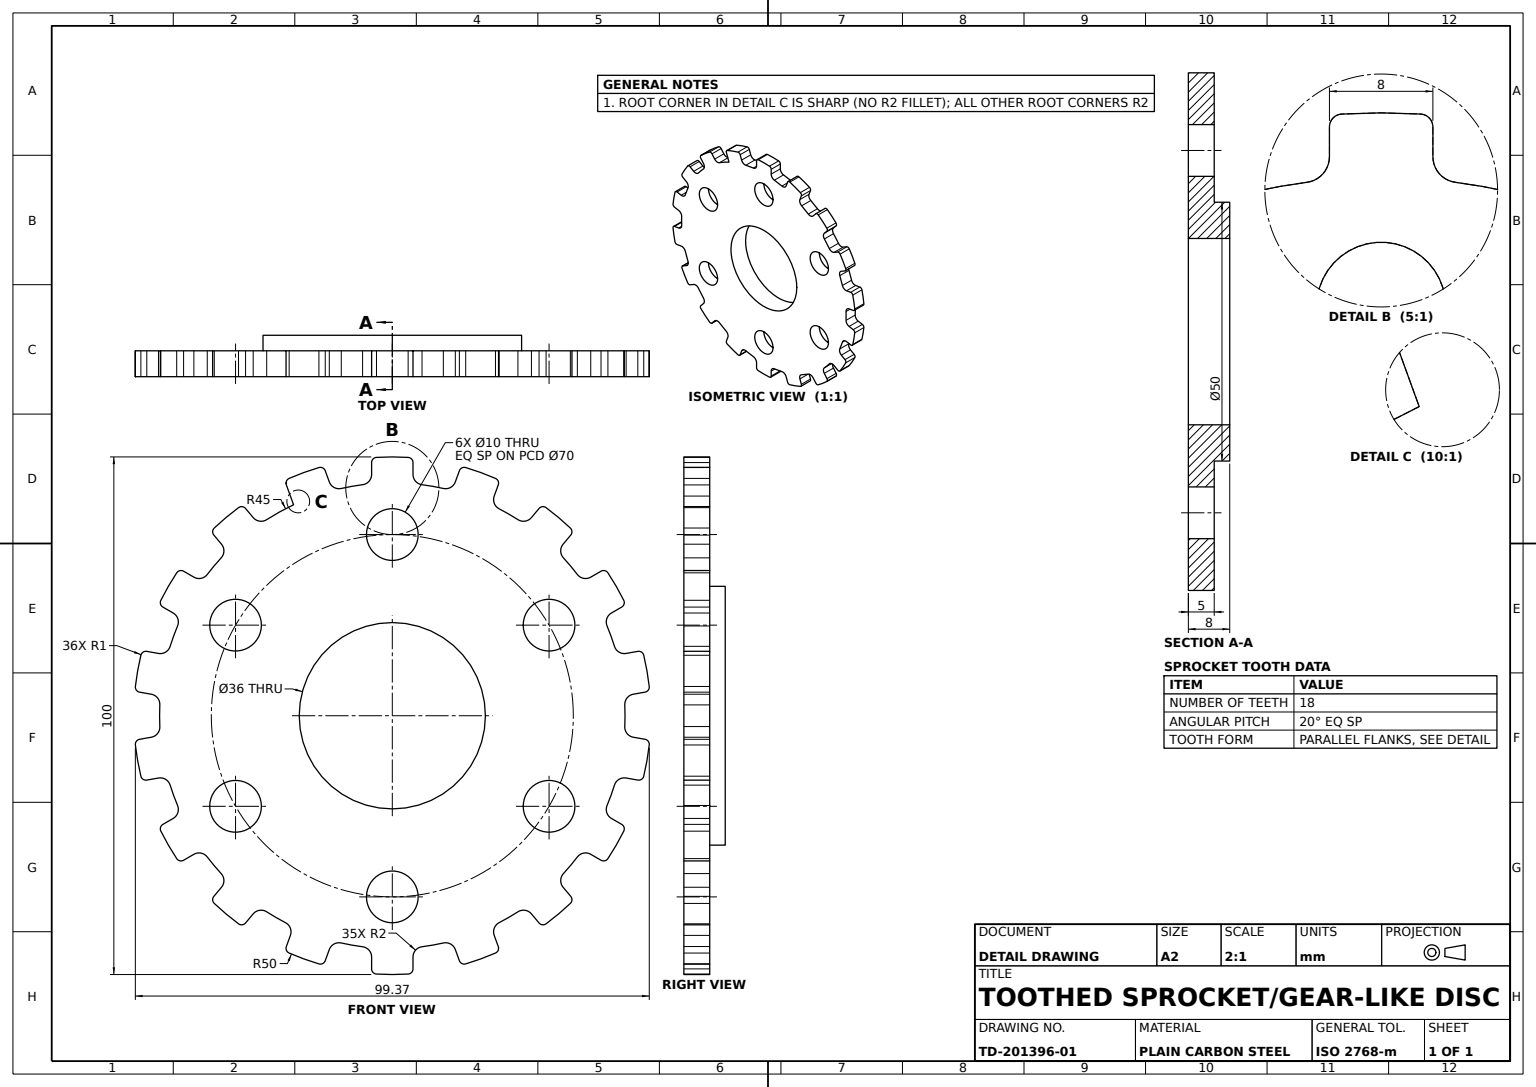
SolidWorks part; units mm, degrees
material "Plain Carbon Steel"
ref_plane "Front Plane" through (0, 0, 0) normal (0, 0, 1) x (1, 0, 0)
ref_plane "Top Plane" through (0, 0, 0) normal (0, 1, 0) x (1, 0, 0)
ref_plane "Right Plane" through (0, 0, 0) normal (1, 0, 0) x (0, 0, -1)
sketch "Sprocket Profile 18T Sketch" plane through (0, 0, 0) normal (0, 0, 1) x (1, 0, 0)
  line L0 (0, 0) -> (0, 50) construction
  line L1 (4, 44.8219) -> (4, 49.8397)
  line L2 (-4, 44.8219) -> (-4, 49.8397)
  line L3 (11.5712, 43.4869) -> (13.2874, 48.2021)
  line L4 (-4, 0) -> (-4, 50) construction
  line L5 (4, 0) -> (4, 50) construction
  line L6 (19.0888, 40.7507) -> (20.805, 45.466)
  line L7 (25.7468, 36.9067) -> (28.9722, 40.7506)
  line L8 (31.8751, 31.7644) -> (35.1005, 35.6083)
  line L9 (36.8169, 25.875) -> (41.1625, 28.384)
  line L10 (40.8169, 18.9468) -> (45.1625, 21.4558)
  line L11 (43.4463, 11.7225) -> (48.388, 12.5938)
  line L12 (44.8355, 3.844) -> (49.7772, 4.7153)
  line L13 (44.8355, -3.844) -> (49.7772, -4.7153)
  line L14 (43.4463, -11.7225) -> (48.388, -12.5938)
  line L15 (40.8169, -18.9468) -> (45.1625, -21.4558)
  line L16 (36.8169, -25.875) -> (41.1625, -28.384)
  line L17 (31.8751, -31.7644) -> (35.1005, -35.6083)
  line L18 (25.7468, -36.9067) -> (28.9722, -40.7506)
  line L19 (19.0888, -40.7507) -> (20.805, -45.466)
  line L20 (11.5712, -43.4869) -> (13.2874, -48.2021)
  line L21 (4, -44.8219) -> (4, -49.8397)
  line L22 (-4, -44.8219) -> (-4, -49.8397)
  line L23 (-11.5712, -43.4869) -> (-13.2874, -48.2021)
  line L24 (-19.0888, -40.7507) -> (-20.805, -45.466)
  line L25 (-25.7468, -36.9067) -> (-28.9722, -40.7506)
  line L26 (-31.8751, -31.7644) -> (-35.1005, -35.6083)
  line L27 (-36.8169, -25.875) -> (-41.1625, -28.384)
  line L28 (-40.8169, -18.9468) -> (-45.1625, -21.4558)
  line L29 (-43.4463, -11.7225) -> (-48.388, -12.5938)
  line L30 (-44.8355, -3.844) -> (-49.7772, -4.7153)
  line L31 (-44.8355, 3.844) -> (-49.7772, 4.7153)
  line L32 (-43.4463, 11.7225) -> (-48.388, 12.5938)
  line L33 (-40.8169, 18.9468) -> (-45.1625, 21.4558)
  line L34 (-36.8169, 25.875) -> (-41.1625, 28.384)
  line L35 (-31.8751, 31.7644) -> (-35.1005, 35.6083)
  line L36 (-25.7468, 36.9067) -> (-28.9722, 40.7506)
  line L37 (-19.0888, 40.7507) -> (-20.805, 45.466)
  line L38 (-11.5712, 43.4869) -> (-13.2874, 48.2021)
  arc A0 (-4, 44.8219) -> (-11.5712, 43.4869) centre (0, 0) ccw
  arc A1 (4, 49.8397) -> (-4, 49.8397) centre (0, 0) ccw
  arc A2 (20.805, 45.466) -> (13.2874, 48.2021) centre (0, 0) ccw
  arc A3 (35.1005, 35.6083) -> (28.9722, 40.7506) centre (0, 0) ccw
  arc A4 (45.1625, 21.4558) -> (41.1625, 28.384) centre (0, 0) ccw
  arc A5 (49.7772, 4.7153) -> (48.388, 12.5938) centre (0, 0) ccw
  arc A6 (48.388, -12.5938) -> (49.7772, -4.7153) centre (0, 0) ccw
  arc A7 (41.1625, -28.384) -> (45.1625, -21.4558) centre (0, 0) ccw
  arc A8 (28.9722, -40.7506) -> (35.1005, -35.6083) centre (0, 0) ccw
  arc A9 (13.2874, -48.2021) -> (20.805, -45.466) centre (0, 0) ccw
  arc A10 (-4, -49.8397) -> (4, -49.8397) centre (0, 0) ccw
  arc A11 (-20.805, -45.466) -> (-13.2874, -48.2021) centre (0, 0) ccw
  arc A12 (-35.1005, -35.6083) -> (-28.9722, -40.7506) centre (0, 0) ccw
  arc A13 (-45.1625, -21.4558) -> (-41.1625, -28.384) centre (0, 0) ccw
  arc A14 (-49.7772, -4.7153) -> (-48.388, -12.5938) centre (0, 0) ccw
  arc A15 (-48.388, 12.5938) -> (-49.7772, 4.7153) centre (0, 0) ccw
  arc A16 (-41.1625, 28.384) -> (-45.1625, 21.4558) centre (0, 0) ccw
  arc A17 (-28.9722, 40.7506) -> (-35.1005, 35.6083) centre (0, 0) ccw
  arc A18 (-13.2874, 48.2021) -> (-20.805, 45.466) centre (0, 0) ccw
  arc A19 (-19.0888, 40.7507) -> (-25.7468, 36.9067) centre (0, 0) ccw
  arc A20 (-31.8751, 31.7644) -> (-36.8169, 25.875) centre (0, 0) ccw
  arc A21 (-40.8169, 18.9468) -> (-43.4463, 11.7225) centre (0, 0) ccw
  arc A22 (-44.8355, 3.844) -> (-44.8355, -3.844) centre (0, 0) ccw
  arc A23 (-43.4463, -11.7225) -> (-40.8169, -18.9468) centre (0, 0) ccw
  arc A24 (-36.8169, -25.875) -> (-31.8751, -31.7644) centre (0, 0) ccw
  arc A25 (-25.7468, -36.9067) -> (-19.0888, -40.7507) centre (0, 0) ccw
  arc A26 (-11.5712, -43.4869) -> (-4, -44.8219) centre (0, 0) ccw
  arc A27 (4, -44.8219) -> (11.5712, -43.4869) centre (0, 0) ccw
  arc A28 (19.0888, -40.7507) -> (25.7468, -36.9067) centre (0, 0) ccw
  arc A29 (31.8751, -31.7644) -> (36.8169, -25.875) centre (0, 0) ccw
  arc A30 (40.8169, -18.9468) -> (43.4463, -11.7225) centre (0, 0) ccw
  arc A31 (44.8355, -3.844) -> (44.8355, 3.844) centre (0, 0) ccw
  arc A32 (11.5712, 43.4869) -> (4, 44.8219) centre (0, 0) ccw
  arc A33 (25.7468, 36.9067) -> (19.0888, 40.7507) centre (0, 0) ccw
  arc A34 (36.8169, 25.875) -> (31.8751, 31.7644) centre (0, 0) ccw
  arc A35 (43.4463, 11.7225) -> (40.8169, 18.9468) centre (0, 0) ccw
  point P82 (0, 0)
  dimension "D1" = 4
  dimension "D4" = 100
  dimension "D5" = 90
  dimension "D3" = 18
  dimension "D2" = 4
extrude "Sprocket Plate 18T" add sketch "Sprocket Profile 18T Sketch" along normal blind 5
sketch "Plate Holes Sketch" plane through (0, 0, 0) normal (0, 0, 1) x (1, 0, 0)
  line L0 (0, 0) -> (0, 35) construction
  circle A0 centre (0, 35) radius 5
  circle A1 centre (30.3109, 17.5) radius 5
  circle A2 centre (30.3109, -17.5) radius 5
  circle A3 centre (0, -35) radius 5
  circle A4 centre (-30.3109, -17.5) radius 5
  circle A5 centre (-30.3109, 17.5) radius 5
  point P16 (0, 0)
  dimension "D1" = 6
  dimension "D2" = 10
  dimension "D3" = 30.3109
extrude "Plate Holes Cut" cut sketch "Plate Holes Sketch" along normal through all
sketch "Back Boss Sketch" plane through (0, 0, 0) normal (0, 0, -1) x (-1, 0, 0)
  circle A0 centre (0, 0) radius 25
  dimension "D1" = 50
extrude "Back Boss 3mm" add sketch "Back Boss Sketch" along normal blind 3
sketch "Back Boss Cut Sketch" plane through (0, 0, -3) normal (0, 0, -1) x (-1, 0, 0)
  circle A0 centre (0, 0) radius 18
  dimension "D1" = 36
extrude "Back Boss Cut" cut sketch "Back Boss Cut Sketch" against normal through all
fillet "Plate Fillet R2" radius 2 35 edges at (40.8169, -18.9468, 2.5) (43.4463, -11.7225, 2.5) (4, -44.8219, 2.5) (11.5712, -43.4869, 2.5) (-4, -44.8219, 2.5) (-11.5712, -43.4869, 2.5) (-19.0888, -40.7507, 2.5) (-25.7468, -36.9067, 2.5) (-31.8751, -31.7644, 2.5) (-36.8169, -25.875, 2.5) (25.7468, 36.9067, 2.5) (11.5712, 43.4869, 2.5) (-4, 44.8219, 2.5) (-31.8751, 31.7644, 2.5) (-40.8169, 18.9468, 2.5) (-44.8355, 3.844, 2.5) (-40.8169, -18.9468, 2.5) (-43.4463, -11.7225, 2.5) (-44.8355, -3.844, 2.5) (-43.4463, 11.7225, 2.5) (-36.8169, 25.875, 2.5) (-25.7468, 36.9067, 2.5) (-11.5712, 43.4869, 2.5) (4, 44.8219, 2.5) (19.0888, 40.7507, 2.5) (31.8751, 31.7644, 2.5) (36.8169, 25.875, 2.5) (40.8169, 18.9468, 2.5) (43.4463, 11.7225, 2.5) (44.8355, 3.844, 2.5) (44.8355, -3.844, 2.5) (19.0888, -40.7507, 2.5) (25.7468, -36.9067, 2.5) (31.8751, -31.7644, 2.5) (36.8169, -25.875, 2.5)
fillet "Plate Fillet R1" radius 1 36 edges at (-20.805, 45.466, 2.5) (-13.2874, 48.2021, 2.5) (-35.1005, 35.6083, 2.5) (-28.9722, 40.7506, 2.5) (-45.1625, 21.4558, 2.5) (-41.1625, 28.384, 2.5) (-48.388, 12.5938, 2.5) (-49.7772, 4.7153, 2.5) (-49.7772, -4.7153, 2.5) (-48.388, -12.5938, 2.5) (-45.1625, -21.4558, 2.5) (-41.1625, -28.384, 2.5) (-35.1005, -35.6083, 2.5) (-28.9722, -40.7506, 2.5) (-20.805, -45.466, 2.5) (-13.2874, -48.2021, 2.5) (-4, -49.8397, 2.5) (4, -49.8397, 2.5) (13.2874, -48.2021, 2.5) (20.805, -45.466, 2.5) (28.9722, -40.7506, 2.5) (35.1005, -35.6083, 2.5) (45.1625, -21.4558, 2.5) (41.1625, -28.384, 2.5) (48.388, -12.5938, 2.5) (49.7772, -4.7153, 2.5) (49.7772, 4.7153, 2.5) (48.388, 12.5938, 2.5) (45.1625, 21.4558, 2.5) (41.1625, 28.384, 2.5) (35.1005, 35.6083, 2.5) (28.9722, 40.7506, 2.5) (20.805, 45.466, 2.5) (13.2874, 48.2021, 2.5) (4, 49.8397, 2.5) (-4, 49.8397, 2.5)
